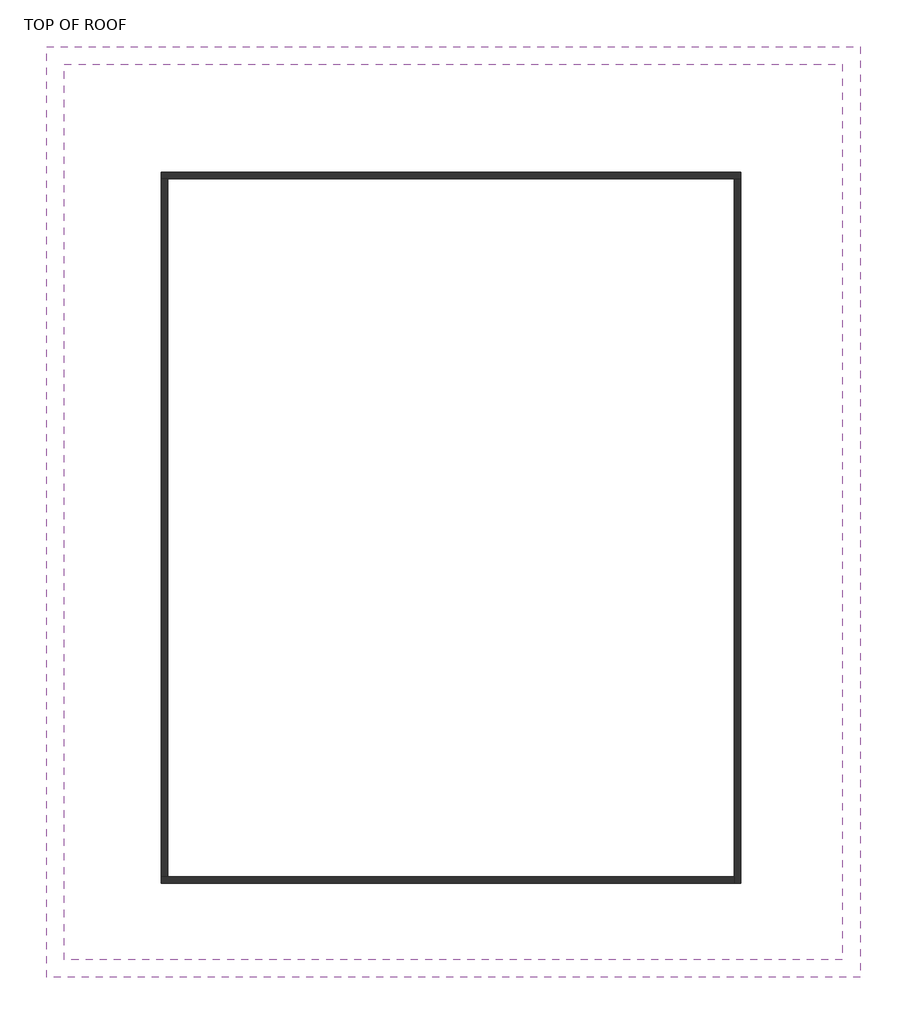
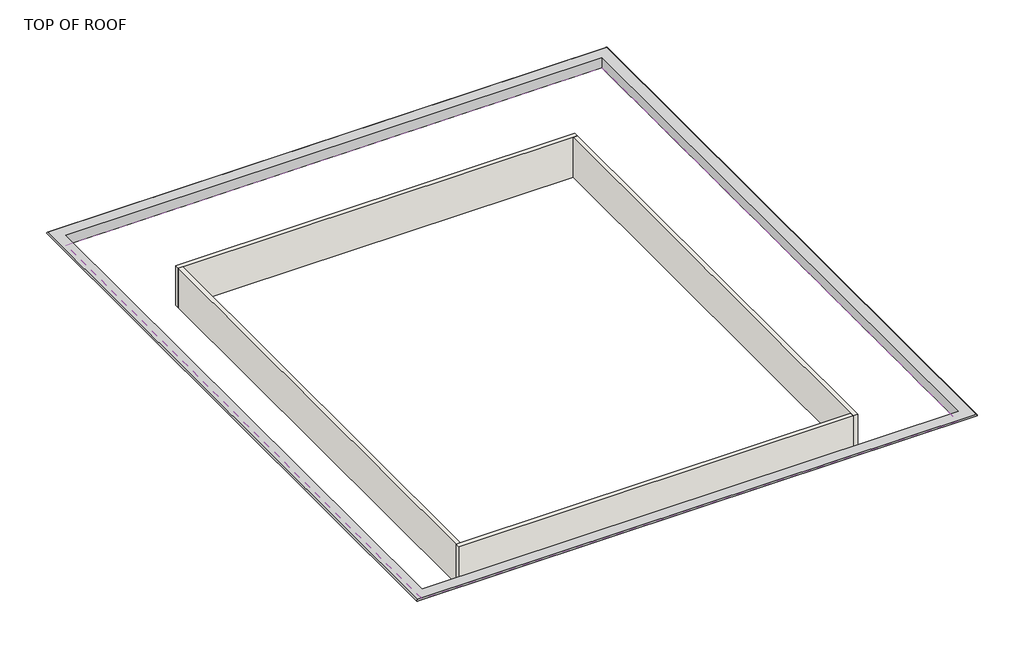
# One storey: 4 walls, 1 proxy, 1 roof.
"""IFC4 building model written with IfcOpenShell, lengths in millimetres."""

from ifc_helpers import new_model, si_unit, frame, origin, place, context, project, spatial, polyline, outline, extrude, faceted_brep, transform, mapped, element, save
from components import generic_models_18_generic_models_18_23725794

model = new_model("IFC4")

# Units and contexts
model_context = context("Model", 3, world=origin())
ifc_project = project(units=[si_unit("LENGTHUNIT", "METRE", prefix="MILLI")], contexts=[model_context])

# Site, building, storey
site = spatial("IfcSite", under=ifc_project)
building = spatial("IfcBuilding", under=site)
storey = spatial("IfcBuildingStorey", under=building, Name="TOP OF ROOF", Elevation=9448.8)

# Proxy
placement = place(None, origin())
generic_models_18_generic_models_18_shape = generic_models_18_generic_models_18_23725794(model_context)
element("IfcBuildingElementProxy", 1, Name="Generic Models 18 : Generic Models 18", ObjectType="Generic Models 18 : Generic Models 18", at=placement, inside=storey, context=model_context, shape_type="MappedRepresentation", body=[
    mapped(generic_models_18_generic_models_18_shape, transform((0.0, 0.0, 0.0), x_axis=(1.0, 0.0, 0.0), y_axis=(0.0, 1.0, 0.0), z_axis=(0.0, 0.0, 1.0))),
])

# Roof
element("IfcRoof", 2, ObjectType="ROOFING 1'", at=placement, inside=storey, context=model_context, shape_type="SweptSolid", body=[
    extrude(outline(polyline([(-11701.9275518, 10386.9473869), (3818.6235854, 10386.9473869), (3818.6235854, -7475.3142532), (-11701.9275518, -7475.3142532), (-11701.9275518, 10386.9473869)])), frame((0.0, 0.0, 10668.0), z_axis=(0.0, 0.0, 1.0), x_axis=(1.0, 0.0, 0.0)), (0.0, 0.0, 1.0), 304.8),
])

# Walls
element("IfcWall", 3, ObjectType="parapet wall 5\"", at=placement, inside=storey, context=model_context, shape_type="Brep", body=[
    faceted_brep([(-9763.9781265, 8107.5857468, 9448.8), (-9636.9781265, 8107.5857468, 9448.8), (1666.0218735, 8107.5857468, 9448.8), (1793.0218735, 8107.5857468, 9448.8), (1793.0218735, 8107.5857468, 10668.0), (1666.0218735, 8107.5857468, 10668.0), (-9636.9781265, 8107.5857468, 10668.0), (-9763.9781265, 8107.5857468, 10668.0), (-9763.9781265, 8234.5857468, 9448.8), (-9763.9781265, 8234.5857468, 10668.0), (1793.0218735, 8234.5857468, 10668.0), (1793.0218735, 8234.5857468, 9448.8)], [[[0, 1, 2, 3, 4, 5, 6, 7]], [[8, 9, 10, 11]], [[3, 2, 1, 0, 8, 11]], [[7, 6, 5, 4, 10, 9]], [[4, 3, 11, 10]], [[0, 7, 9, 8]]]),
])
element("IfcWall", 4, ObjectType="parapet wall 5\"", at=placement, inside=storey, context=model_context, shape_type="Brep", body=[
    faceted_brep([(1666.0218735, 8107.5857468, 9448.8), (1666.0218735, -5951.3142532, 9448.8), (1666.0218735, -5951.3142532, 9496.7382261), (1666.0218735, -5951.3142532, 10668.0), (1666.0218735, -5824.3142532, 10668.0), (1666.0218735, 8107.5857468, 10668.0), (1793.0218735, 8107.5857468, 9448.8), (1793.0218735, 8107.5857468, 10668.0), (1793.0218735, -5951.3142532, 10668.0), (1793.0218735, -5951.3142532, 9448.8)], [[[0, 1, 2, 3, 4, 5]], [[6, 7, 8, 9]], [[1, 0, 6, 9]], [[5, 4, 3, 8, 7]], [[0, 5, 7, 6]], [[3, 2, 1, 9, 8]]]),
])
element("IfcWall", 5, ObjectType="parapet wall 5\"", at=placement, inside=storey, context=model_context, shape_type="Brep", body=[
    faceted_brep([(1666.0218735, -5824.3142532, 9496.7382261), (-9763.9781265, -5824.3142532, 9496.7382261), (-9763.9781265, -5824.3142532, 10668.0), (-9636.9781265, -5824.3142532, 10668.0), (1666.0218735, -5824.3142532, 10668.0), (1666.0218735, -5951.3142532, 9496.7382261), (1666.0218735, -5951.3142532, 10668.0), (-9763.9781265, -5951.3142532, 10668.0), (-9763.9781265, -5951.3142532, 9496.7382261)], [[[0, 1, 2, 3, 4]], [[5, 6, 7, 8]], [[1, 0, 5, 8]], [[4, 3, 2, 7, 6]], [[0, 4, 6, 5]], [[2, 1, 8, 7]]]),
])
element("IfcWall", 6, ObjectType="parapet wall 5\"", at=placement, inside=storey, context=model_context, shape_type="Brep", body=[
    faceted_brep([(-9636.9781265, -5824.3142532, 9448.8), (-9636.9781265, 8107.5857468, 9448.8), (-9636.9781265, 8107.5857468, 10668.0), (-9636.9781265, -5824.3142532, 10668.0), (-9763.9781265, -5824.3142532, 9448.8), (-9763.9781265, -5824.3142532, 9496.7382261), (-9763.9781265, -5824.3142532, 10668.0), (-9763.9781265, 8107.5857468, 10668.0), (-9763.9781265, 8107.5857468, 9448.8)], [[[0, 1, 2, 3]], [[4, 5, 6, 7, 8]], [[1, 0, 4, 8]], [[3, 2, 7, 6]], [[2, 1, 8, 7]], [[0, 3, 6, 5, 4]]]),
])

save(model, "model.ifc")

# Revit data of these elements
# Type "ROOFING 1'"
#   Assembly Code = "B1020"
# Type "parapet wall 5\""
#   Assembly Code = "B2010"
# Element 1 (IfcBuildingElementProxy, "Generic Models 18 : Generic Models 18")
#   Phase Created = New Construction
# Element 2 (IfcRoof, "ROOFING 1'")
#   built-in parameter 1001705 = 36 (stored number, unit not read)
#   built-in parameter 1001701 = 4 (stored number, unit not read)
#   built-in parameter 1001710 = 33615
#   Phase Created = New Construction
# Elements 3, 4, 6 (IfcWall, "parapet wall 5\"")
#   Top Offset = 0' - 0"
#   Base Offset = 0' - 0"
#   Unconnected Height = 4' - 0"
#   wall height = 4' - 0"
#   Phase Created = New Construction
#   Base Constraint = TOP OF ROOF
# Element 5 (IfcWall, "parapet wall 5\"")
#   built-in parameter 1001111 = 0' - 1.88733"
#   Top Offset = 0' - 0"
#   Base Offset = 0' - 1.88733"
#   Unconnected Height = 3' - 10.11267"
#   wall height = 3' - 10.11267"
#   Phase Created = New Construction
#   Base Constraint = TOP OF ROOF
